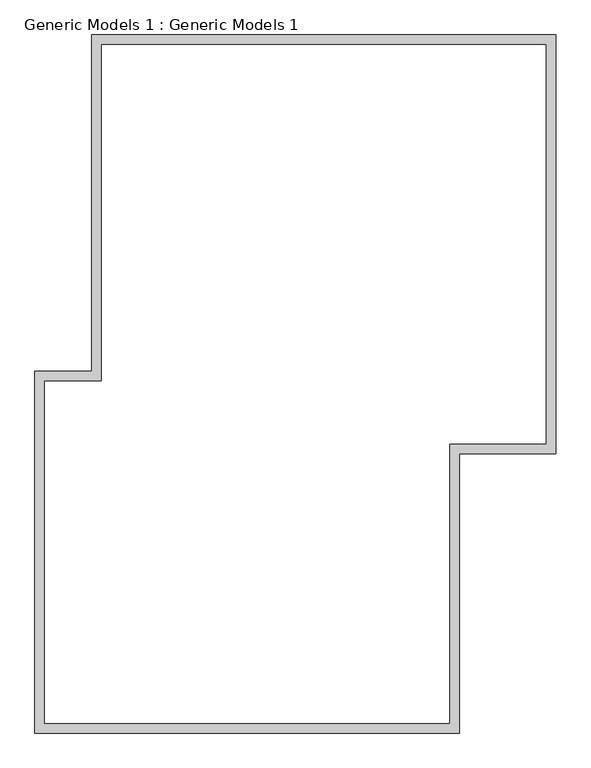
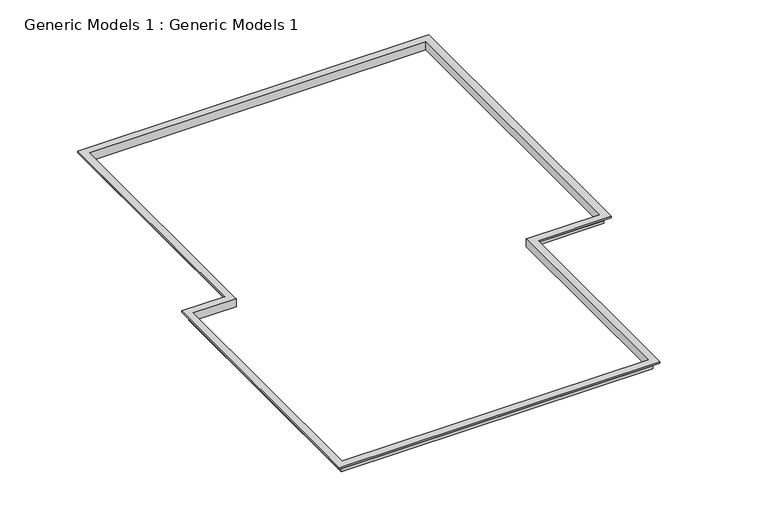
"""IFC4 building model written with IfcOpenShell, lengths in millimetres: proxy geometry, Generic Models 1 : Generic Models 1."""

from ifc_helpers import new_model, si_unit, frame, origin, place, context, project, spatial, polyline, ellipse_curve, source, transform, mapped, element, save
from ifc_brep_helpers import plane_surface, revolved_surface, advanced_brep


def generic_models_1_generic_models_1_7431621c(model_context):
    return source(origin(), model_context, "Body", "AdvancedBrep", [
        advanced_brep(
        [(-912.3415084, 8678.933346, 16002.0), (-912.3415084, 8678.933346, 15849.6), (-912.3415084, 3344.933346, 15849.6), (-912.3415084, 3344.933346, 16002.0), (-778.9915084, 8812.283346, 15974.4426131), (-778.9915084, 8812.283346, 16002.0), (-778.9915084, 3211.583346, 16002.0), (-778.9915084, 3211.583346, 15974.4426131), (-804.3915084, 8786.883346, 15955.3926131), (-804.3915084, 8786.883346, 15974.4426131), (-804.3915084, 3236.983346, 15974.4426131), (-804.3915084, 3236.983346, 15955.3926131), (-861.5415084, 8729.733346, 15900.4), (-829.7915084, 8761.483346, 15955.3926131), (-829.7915084, 3262.383346, 15955.3926131), (-861.5415084, 3294.133346, 15900.4), (-861.5415084, 8729.733346, 15849.6), (-861.5415084, 3294.133346, 15849.6), (-2207.7415084, 3344.933346, 15849.6), (-2207.7415084, 3344.933346, 16002.0), (-2074.3915084, 3211.583346, 16002.0), (-2074.3915084, 3211.583346, 15974.4426131), (-2099.7915084, 3236.983346, 15974.4426131), (-2099.7915084, 3236.983346, 15955.3926131), (-2125.1915084, 3262.383346, 15955.3926131), (-2156.9415084, 3294.133346, 15900.4), (-2156.9415084, 3294.133346, 15849.6), (-2207.7415084, -388.866654, 15849.6), (-2207.7415084, -388.866654, 16002.0), (-2074.3915084, -522.216654, 16002.0), (-2074.3915084, -522.216654, 15974.4426131), (-2099.7915084, -496.816654, 15974.4426131), (-2099.7915084, -496.816654, 15955.3926131), (-2125.1915084, -471.416654, 15955.3926131), (-2156.9415084, -439.666654, 15900.4), (-2156.9415084, -439.666654, 15849.6), (-7617.9415084, -388.866654, 15849.6), (-7617.9415084, -388.866654, 16002.0), (-7751.2915084, -522.216654, 16002.0), (-7751.2915084, -522.216654, 15974.4426131), (-7725.8915084, -496.816654, 15974.4426131), (-7725.8915084, -496.816654, 15955.3926131), (-7700.4915084, -471.416654, 15955.3926131), (-7668.7415084, -439.666654, 15900.4), (-7668.7415084, -439.666654, 15849.6), (-7617.9415084, 4183.133346, 15849.6), (-7617.9415084, 4183.133346, 16002.0), (-7751.2915084, 4316.483346, 16002.0), (-7751.2915084, 4316.483346, 15974.4426131), (-7725.8915084, 4291.083346, 15974.4426131), (-7725.8915084, 4291.083346, 15955.3926131), (-7700.4915084, 4265.683346, 15955.3926131), (-7668.7415084, 4233.933346, 15900.4), (-7668.7415084, 4233.933346, 15849.6), (-6855.9415084, 4183.133346, 15849.6), (-6855.9415084, 4183.133346, 16002.0), (-6989.2915084, 4316.483346, 16002.0), (-6989.2915084, 4316.483346, 15974.4426131), (-6963.8915084, 4291.083346, 15974.4426131), (-6963.8915084, 4291.083346, 15955.3926131), (-6938.4915084, 4265.683346, 15955.3926131), (-6906.7415084, 4233.933346, 15900.4), (-6906.7415084, 4233.933346, 15849.6), (-6855.9415084, 8678.933346, 15849.6), (-6855.9415084, 8678.933346, 16002.0), (-6989.2915084, 8812.283346, 16002.0), (-6989.2915084, 8812.283346, 15974.4426131), (-6963.8915084, 8786.883346, 15974.4426131), (-6963.8915084, 8786.883346, 15955.3926131), (-6938.4915084, 8761.483346, 15955.3926131), (-6906.7415084, 8729.733346, 15900.4), (-6906.7415084, 8729.733346, 15849.6)],
        [
            (0, 1),
            (1, 2),
            (2, 3),
            (3, 0),
            (4, 5),
            (5, 6),
            (6, 7),
            (7, 4),
            (8, 9),
            (9, 10),
            (10, 11),
            (11, 8),
            (12, 13, ellipse_curve(frame((-798.0415084, 8793.233346, 15900.4), z_axis=(-0.7071067811865456, 0.7071067811865495, 0.0), x_axis=(-0.7071067811865495, -0.7071067811865456, 0.0)), 89.8025612, 63.5)),
            (13, 14),
            (14, 15, ellipse_curve(frame((-798.0415084, 3230.633346, 15900.4), z_axis=(-0.7071067811865496, -0.7071067811865454, 0.0), x_axis=(0.7071067811865452, -0.7071067811865497, 0.0)), 89.8025612, 63.5)),
            (15, 12),
            (16, 12),
            (15, 17),
            (17, 16),
            (2, 18),
            (18, 19),
            (19, 3),
            (6, 20),
            (20, 21),
            (21, 7),
            (10, 22),
            (22, 23),
            (23, 11),
            (14, 24),
            (24, 25, ellipse_curve(frame((-2093.4415084, 3230.633346, 15900.4), z_axis=(-0.7071067811865496, -0.7071067811865455, 0.0), x_axis=(-0.7071067811865455, 0.7071067811865496, 0.0)), 89.8025612, 63.5)),
            (25, 15),
            (25, 26),
            (26, 17),
            (18, 27),
            (27, 28),
            (28, 19),
            (20, 29),
            (29, 30),
            (30, 21),
            (22, 31),
            (31, 32),
            (32, 23),
            (24, 33),
            (33, 34, ellipse_curve(frame((-2093.4415084, -503.166654, 15900.4), z_axis=(-0.7071067811865495, -0.7071067811865456, 0.0), x_axis=(0.7071067811865455, -0.7071067811865495, 0.0)), 89.8025612, 63.5)),
            (34, 25),
            (34, 35),
            (35, 26),
            (27, 36),
            (36, 37),
            (37, 28),
            (29, 38),
            (38, 39),
            (39, 30),
            (31, 40),
            (40, 41),
            (41, 32),
            (33, 42),
            (42, 43, ellipse_curve(frame((-7732.2415084, -503.166654, 15900.4), z_axis=(-0.7071067811865457, 0.7071067811865495, 0.0), x_axis=(-0.7071067811865493, -0.7071067811865457, 0.0)), 89.8025612, 63.5)),
            (43, 34),
            (43, 44),
            (44, 35),
            (36, 45),
            (45, 46),
            (46, 37),
            (38, 47),
            (47, 48),
            (48, 39),
            (40, 49),
            (49, 50),
            (50, 41),
            (42, 51),
            (51, 52, ellipse_curve(frame((-7732.2415084, 4297.433346, 15900.4), z_axis=(0.7071067811865493, 0.7071067811865456, 0.0), x_axis=(-0.7071067811865456, 0.7071067811865496, 0.0)), 89.8025612, 63.5)),
            (52, 43),
            (52, 53),
            (53, 44),
            (45, 54),
            (54, 55),
            (55, 46),
            (47, 56),
            (56, 57),
            (57, 48),
            (49, 58),
            (58, 59),
            (59, 50),
            (51, 60),
            (60, 61, ellipse_curve(frame((-6970.2415084, 4297.433346, 15900.4), z_axis=(0.7071067811865493, 0.7071067811865457, 0.0), x_axis=(0.7071067811865457, -0.7071067811865495, 0.0)), 89.8025612, 63.5)),
            (61, 52),
            (61, 62),
            (62, 53),
            (54, 63),
            (63, 64),
            (64, 55),
            (56, 65),
            (65, 66),
            (66, 57),
            (58, 67),
            (67, 68),
            (68, 59),
            (60, 69),
            (69, 70, ellipse_curve(frame((-6970.2415084, 8793.233346, 15900.4), z_axis=(0.7071067811865492, 0.7071067811865458, 0.0), x_axis=(-0.7071067811865457, 0.7071067811865492, 0.0)), 89.8025612, 63.5)),
            (70, 61),
            (70, 71),
            (71, 62),
            (71, 16),
            (1, 63),
            (0, 64),
            (5, 65),
            (4, 66),
            (9, 67),
            (8, 68),
            (13, 69),
            (12, 70),
        ],
        [
            plane_surface(frame((-912.3415084, 8678.933346, 15849.6), z_axis=(-1.0, 0.0, 0.0), x_axis=(0.0, -1.0, 0.0))),
            plane_surface(frame((-778.9915084, 8812.283346, 16002.0), z_axis=(1.0, 0.0, 0.0), x_axis=(0.0, -1.0, 0.0))),
            plane_surface(frame((-804.3915084, 8786.883346, 15974.4426131), z_axis=(1.0, 0.0, 0.0), x_axis=(0.0, -1.0, 0.0))),
            revolved_surface(polyline([(-861.5415084, 3167.1333460075602, 15900.4), (-861.5415084, 8856.733345992441, 15900.4)]), (-798.0415084, 8678.933346, 15900.4), (0.0, -1.0, 0.0)),
            plane_surface(frame((-861.5415084, 8729.733346, 15900.4), z_axis=(1.0, 0.0, 0.0), x_axis=(0.0, -1.0, 0.0))),
            plane_surface(frame((-912.3415084, 3344.933346, 15849.6), z_axis=(0.0, 1.0, 0.0), x_axis=(-1.0, 0.0, 0.0))),
            plane_surface(frame((-778.9915084, 3211.583346, 16002.0), z_axis=(0.0, -1.0, 0.0), x_axis=(-1.0, 0.0, 0.0))),
            plane_surface(frame((-804.3915084, 3236.983346, 15974.4426131), z_axis=(0.0, -1.0, 0.0), x_axis=(-1.0, 0.0, 0.0))),
            revolved_surface(polyline([(-2156.9415084, 3294.133346, 15900.4), (-734.5415084075603, 3294.133346, 15900.4)]), (-912.3415084, 3230.633346, 15900.4), (-1.0, 0.0, 0.0)),
            plane_surface(frame((-861.5415084, 3294.133346, 15900.4), z_axis=(0.0, -1.0, 0.0), x_axis=(-1.0, 0.0, 0.0))),
            plane_surface(frame((-2207.7415084, 3344.933346, 15849.6), z_axis=(-1.0, 0.0, 0.0), x_axis=(0.0, -1.0, 0.0))),
            plane_surface(frame((-2074.3915084, 3211.583346, 16002.0), z_axis=(1.0, 0.0, 0.0), x_axis=(0.0, -1.0, 0.0))),
            plane_surface(frame((-2099.7915084, 3236.983346, 15974.4426131), z_axis=(1.0, 0.0, 0.0), x_axis=(0.0, -1.0, 0.0))),
            revolved_surface(polyline([(-2156.9415084, -566.6666539924404, 15900.4), (-2156.9415084, 3294.133346, 15900.4)]), (-2093.4415084, 3344.933346, 15900.4), (0.0, -1.0, 0.0)),
            plane_surface(frame((-2156.9415084, 3294.133346, 15900.4), z_axis=(1.0, 0.0, 0.0), x_axis=(0.0, -1.0, 0.0))),
            plane_surface(frame((-2207.7415084, -388.866654, 15849.6), z_axis=(0.0, 1.0, 0.0), x_axis=(-1.0, 0.0, 0.0))),
            plane_surface(frame((-2074.3915084, -522.216654, 16002.0), z_axis=(0.0, -1.0, 0.0), x_axis=(-1.0, 0.0, 0.0))),
            plane_surface(frame((-2099.7915084, -496.816654, 15974.4426131), z_axis=(0.0, -1.0, 0.0), x_axis=(-1.0, 0.0, 0.0))),
            revolved_surface(polyline([(-7795.741508392441, -439.666654, 15900.4), (-2029.9415084075604, -439.666654, 15900.4)]), (-2207.7415084, -503.166654, 15900.4), (-1.0, 0.0, 0.0)),
            plane_surface(frame((-2156.9415084, -439.666654, 15900.4), z_axis=(0.0, -1.0, 0.0), x_axis=(-1.0, 0.0, 0.0))),
            plane_surface(frame((-7617.9415084, -388.866654, 15849.6), z_axis=(1.0, 0.0, 0.0), x_axis=(0.0, 1.0, 0.0))),
            plane_surface(frame((-7751.2915084, -522.216654, 16002.0), z_axis=(-1.0, 0.0, 0.0), x_axis=(0.0, 1.0, 0.0))),
            plane_surface(frame((-7725.8915084, -496.816654, 15974.4426131), z_axis=(-1.0, 0.0, 0.0), x_axis=(0.0, 1.0, 0.0))),
            revolved_surface(polyline([(-7668.7415084, 4360.93334599244, 15900.4), (-7668.7415084, -566.6666539924397, 15900.4)]), (-7732.2415084, -388.866654, 15900.4), (0.0, 1.0, 0.0)),
            plane_surface(frame((-7668.7415084, -439.666654, 15900.4), z_axis=(-1.0, 0.0, 0.0), x_axis=(0.0, 1.0, 0.0))),
            plane_surface(frame((-7617.9415084, 4183.133346, 15849.6), z_axis=(0.0, -1.0, 0.0), x_axis=(1.0, 0.0, 0.0))),
            plane_surface(frame((-7751.2915084, 4316.483346, 16002.0), z_axis=(0.0, 1.0, 0.0), x_axis=(1.0, 0.0, 0.0))),
            plane_surface(frame((-7725.8915084, 4291.083346, 15974.4426131), z_axis=(0.0, 1.0, 0.0), x_axis=(1.0, 0.0, 0.0))),
            revolved_surface(polyline([(-6906.7415084, 4233.933346, 15900.4), (-7795.74150839244, 4233.933346, 15900.4)]), (-7617.9415084, 4297.433346, 15900.4), (1.0, 0.0, 0.0)),
            plane_surface(frame((-7668.7415084, 4233.933346, 15900.4), z_axis=(0.0, 1.0, 0.0), x_axis=(1.0, 0.0, 0.0))),
            plane_surface(frame((-6855.9415084, 4183.133346, 15849.6), z_axis=(1.0, 0.0, 0.0), x_axis=(0.0, 1.0, 0.0))),
            plane_surface(frame((-6989.2915084, 4316.483346, 16002.0), z_axis=(-1.0, 0.0, 0.0), x_axis=(0.0, 1.0, 0.0))),
            plane_surface(frame((-6963.8915084, 4291.083346, 15974.4426131), z_axis=(-1.0, 0.0, 0.0), x_axis=(0.0, 1.0, 0.0))),
            revolved_surface(polyline([(-6906.7415084, 8856.733345992441, 15900.4), (-6906.7415084, 4233.933346, 15900.4)]), (-6970.2415084, 4183.133346, 15900.4), (0.0, 1.0, 0.0)),
            plane_surface(frame((-6906.7415084, 4233.933346, 15900.4), z_axis=(-1.0, 0.0, 0.0), x_axis=(0.0, 1.0, 0.0))),
            plane_surface(frame((-6906.7415084, 8729.733346, 15849.6), z_axis=(0.0, 0.0, -1.0), x_axis=(1.0, 0.0, 0.0))),
            plane_surface(frame((-6855.9415084, 8678.933346, 15849.6), z_axis=(0.0, -1.0, 0.0), x_axis=(1.0, 0.0, 0.0))),
            plane_surface(frame((-6855.9415084, 8678.933346, 16002.0), z_axis=(0.0, 0.0, 1.0), x_axis=(1.0, 0.0, 0.0))),
            plane_surface(frame((-6989.2915084, 8812.283346, 16002.0), z_axis=(0.0, 1.0, 0.0), x_axis=(1.0, 0.0, 0.0))),
            plane_surface(frame((-6989.2915084, 8812.283346, 15974.4426131), z_axis=(0.0, 0.0, -1.0), x_axis=(1.0, 0.0, 0.0))),
            plane_surface(frame((-6963.8915084, 8786.883346, 15974.4426131), z_axis=(0.0, 1.0, 0.0), x_axis=(1.0, 0.0, 0.0))),
            plane_surface(frame((-6963.8915084, 8786.883346, 15955.3926131), z_axis=(0.0, 0.0, -1.0), x_axis=(1.0, 0.0, 0.0))),
            revolved_surface(polyline([(-734.5415084075594, 8729.733346, 15900.4), (-7033.74150839244, 8729.733346, 15900.4)]), (-6855.9415084, 8793.233346, 15900.4), (1.0, 0.0, 0.0)),
            plane_surface(frame((-6906.7415084, 8729.733346, 15900.4), z_axis=(0.0, 1.0, 0.0), x_axis=(1.0, 0.0, 0.0))),
        ],
        [
            (0, [[1, 2, 3, 4]]),
            (1, [[5, 6, 7, 8]]),
            (2, [[9, 10, 11, 12]]),
            (3, [[13, 14, 15, 16]]),
            (4, [[17, -16, 18, 19]]),
            (5, [[-3, 20, 21, 22]]),
            (6, [[-7, 23, 24, 25]]),
            (7, [[-11, 26, 27, 28]]),
            (8, [[-15, 29, 30, 31]]),
            (9, [[-18, -31, 32, 33]]),
            (10, [[-21, 34, 35, 36]]),
            (11, [[-24, 37, 38, 39]]),
            (12, [[-27, 40, 41, 42]]),
            (13, [[-30, 43, 44, 45]]),
            (14, [[-32, -45, 46, 47]]),
            (15, [[-35, 48, 49, 50]]),
            (16, [[-38, 51, 52, 53]]),
            (17, [[-41, 54, 55, 56]]),
            (18, [[-44, 57, 58, 59]]),
            (19, [[-46, -59, 60, 61]]),
            (20, [[-49, 62, 63, 64]]),
            (21, [[-52, 65, 66, 67]]),
            (22, [[-55, 68, 69, 70]]),
            (23, [[-58, 71, 72, 73]]),
            (24, [[-60, -73, 74, 75]]),
            (25, [[-63, 76, 77, 78]]),
            (26, [[-66, 79, 80, 81]]),
            (27, [[-69, 82, 83, 84]]),
            (28, [[-72, 85, 86, 87]]),
            (29, [[-74, -87, 88, 89]]),
            (30, [[-77, 90, 91, 92]]),
            (31, [[-80, 93, 94, 95]]),
            (32, [[-83, 96, 97, 98]]),
            (33, [[-86, 99, 100, 101]]),
            (34, [[-88, -101, 102, 103]]),
            (35, [[-89, -103, 104, -19, -33, -47, -61, -75], [105, -90, -76, -62, -48, -34, -20, -2]]),
            (36, [[-91, -105, -1, 106]]),
            (37, [[107, -93, -79, -65, -51, -37, -23, -6], [-78, -92, -106, -4, -22, -36, -50, -64]]),
            (38, [[-94, -107, -5, 108]]),
            (39, [[-81, -95, -108, -8, -25, -39, -53, -67], [109, -96, -82, -68, -54, -40, -26, -10]]),
            (40, [[-97, -109, -9, 110]]),
            (41, [[-84, -98, -110, -12, -28, -42, -56, -70], [111, -99, -85, -71, -57, -43, -29, -14]]),
            (42, [[-100, -111, -13, 112]]),
            (43, [[-102, -112, -17, -104]]),
        ],
    ),
    ])


if __name__ == "__main__":
    model = new_model("IFC4")
    model_context = context("Model", 3, world=origin())
    ifc_project = project(units=[si_unit("LENGTHUNIT", "METRE", prefix="MILLI")], contexts=[model_context])
    site = spatial("IfcSite", under=ifc_project)
    building = spatial("IfcBuilding", under=site)
    placement = place(None, origin())
    generic_models_1_generic_models_1_shape = generic_models_1_generic_models_1_7431621c(model_context)
    element("IfcBuildingElementProxy", 1, Name="Generic Models 1 : Generic Models 1", ObjectType="Generic Models 1 : Generic Models 1", at=placement, inside=building, context=model_context, shape_type="MappedRepresentation", body=[
        mapped(generic_models_1_generic_models_1_shape, transform((0.0, 0.0, 0.0), x_axis=(1.0, 0.0, 0.0), y_axis=(0.0, 1.0, 0.0), z_axis=(0.0, 0.0, 1.0))),
    ])
    save(model, "model.ifc")
